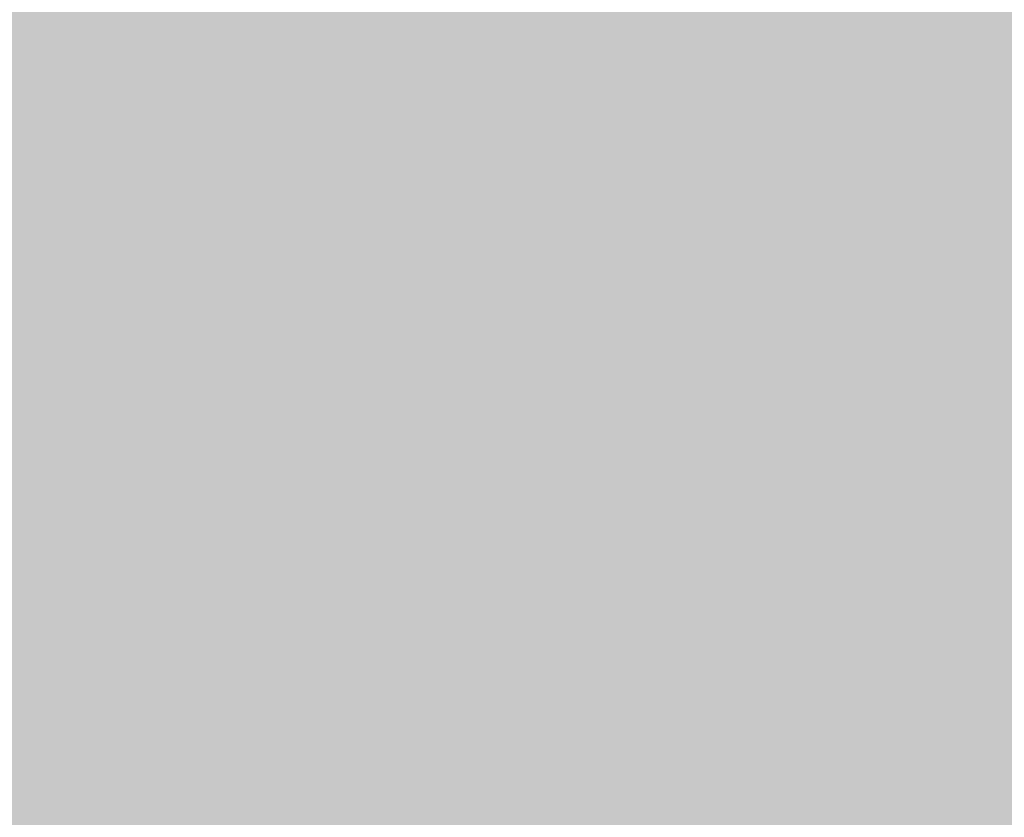
# Model space of a CAD drawing. Units: millimetres. Extents: x 0 to 2267, y 0 to 1823.
# Tile 131 of 256: x 1600.37 to 1611.04, y 1234.76 to 1243.41. Entities that reach past the tile are written whole.
import ezdxf

# ---------------------------------------------------------------- set-up
doc = ezdxf.new("R2010")
doc.units = ezdxf.units.MM
doc.header["$MEASUREMENT"] = 0
doc.layers.add('M-DIMS', color=2, linetype='Continuous', lineweight=25)
doc.layers.add('M-HATC', color=252, linetype='Continuous', lineweight=18)
doc.styles.get("Standard").update_dxf_attribs({"font": 'arial.ttf'})
doc.dimstyles.get("Standard").update_dxf_attribs({"dimtxt": 7, "dimasz": 4, "dimexe": 0.18, "dimexo": 0.0625, "dimgap": 0.09, "dimtad": 0, "dimdec": 0, "dimzin": 0, "dimdsep": 46, "dimtxsty": 'Standard', "dimcen": 0.09, "dimadec": 0, "dimazin": 0, "dimtfac": 1, "dimtdec": 0, "dimtofl": 0, "dimtmove": 0, "dimatfit": 3, "dimfxl": 1, "dimtolj": 1, "dimtzin": 0, "dimarcsym": 0})

# ---------------------------------------------------------------- blocks, each defined once
blk = doc.blocks.new('*D19')
at = {"layer": 'Defpoints', "color": 0, "transparency": 16777216}
for p in [(1605.34, 1483.304), (1445.529, 1333.885)]:
    blk.add_point(p, dxfattribs=at)
at = {"layer": 'M-DIMS', "color": 0, "lineweight": -2, "transparency": 16777216}
for p, q in [((1605.34, 1483.214), (1605.34, 1483.394)), ((1605.25, 1483.304), (1605.43, 1483.304)), ((1366.324, 1259.831), (1442.607, 1331.153))]:
    blk.add_line(p, q, dxfattribs=at)
at = {"layer": 'M-DIMS', "color": 0, "transparency": 16777216}
blk.add_solid([(1442.152, 1331.64), (1443.063, 1330.666), (1445.529, 1333.885)], dxfattribs=at)
at = {"layer": 'M-DIMS', "color": 0, "transparency": 16777216, "insert": (1349.643, 1244.233), "char_height": 7, "attachment_point": 5, "rotation": 43.0753}
blk.add_mtext('\\A1;2X R218.8', dxfattribs=at)

msp = doc.modelspace()

# ---------------------------------------------------------------- hatches: boundary and pattern name
at = {"layer": 'M-HATC'}
h = msp.add_hatch(color=256, dxfattribs=at)
h.dxf.hatch_style = 1
h.paths.add_polyline_path([(2065.771, 1618.062, 0.236068), (2055.771, 1638.062), (1381.087, 1638.062, 0.236068), (1371.087, 1618.062), (1371.087, 1603.062), (2055.771, 1603.062), (2065.771, 1603.062)])
h.paths.add_polyline_path([(2062.772, 1550.296), (2062.772, 1560.296), (1374.086, 1560.296), (1374.086, 1550.296), (1374.086, 1540.296), (1384.086, 1540.296), (1389.086, 1540.296), (2062.772, 1540.296)])
h.paths.add_polyline_path([(1930.929, 1282.766), (1505.929, 1282.766), (1587.628, 1235.597, 0.131652), (1600.128, 1232.247), (1836.73, 1232.247, 0.131652), (1849.23, 1235.597)])
h.paths.add_polyline_path([(1930.929, 1117.417), (1905.929, 1117.417), (1505.929, 1117.417), (1505.929, 1077.417), (1930.929, 1077.417)])
h = msp.add_hatch(color=256, dxfattribs=at)
h.dxf.hatch_style = 1
h.paths.add_polyline_path([(2055.771, 1603.062), (1381.087, 1603.062), (1381.087, 1598.062), (2055.771, 1598.062)])
h.paths.add_polyline_path([(2055.771, 1598.062), (1381.087, 1598.062), (1381.087, 1593.062), (2055.771, 1593.062)])
h.paths.add_polyline_path([(2051.307, 1536.761), (1385.55, 1536.761), (1385.55, 1526.761), (1387.55, 1526.761), (1388.537, 1525.053), (1385.332, 1521.233), (1385.332, 1521.223), (2050.254, 1522.749), (2048.321, 1525.053), (2049.307, 1526.761), (2051.307, 1526.761)])
edge = h.paths.add_edge_path()
edge.add_arc((1847.535, 1379.149), 135, 222.60306, 222.89085, ccw=False)
edge.add_line((1748.166, 1287.766), (1683.092, 1287.766))
edge.add_arc((1583.724, 1379.149), 135, 317.10915, 317.39694, ccw=False)
edge.add_arc((1678.969, 1290.671), 5, 222.8909, 317.1091, ccw=False)
edge.add_arc((1774.213, 1379.149), 135, 222.60306, 222.89085, ccw=False)
edge.add_line((1674.845, 1287.766), (1609.771, 1287.766))
edge.add_arc((1510.403, 1379.149), 135, 317.10915, 317.39694, ccw=False)
edge.add_arc((1605.647, 1290.671), 5, 222.8909, 317.1091, ccw=False)
edge.add_arc((1700.892, 1379.149), 135, 222.60306, 222.89085, ccw=False)
edge.add_line((1601.524, 1287.766), (1536.45, 1287.766))
edge.add_arc((1437.081, 1379.149), 135, 317.10915, 317.39694, ccw=False)
edge.add_arc((1532.326, 1290.671), 5, 222.8909, 317.1091, ccw=False)
edge.add_arc((1627.571, 1379.149), 135, 222.60306, 222.89085, ccw=False)
edge.add_line((1528.203, 1287.766), (1505.929, 1287.766))
edge.add_spline(control_points=[(1505.929, 1287.766), (1504.262, 1287.766), (1504.262, 1282.766), (1505.929, 1282.766)], knot_values=[0, 0, 0, 0, 5, 5, 5, 5], degree=3, periodic=0)
edge.add_line((1505.929, 1282.766), (1930.929, 1282.766))
edge.add_spline(control_points=[(1930.929, 1282.766), (1932.596, 1282.766), (1932.596, 1287.766), (1930.929, 1287.766)], knot_values=[0, 0, 0, 0, 5, 5, 5, 5], degree=3, periodic=0)
edge.add_line((1930.929, 1287.766), (1903.056, 1287.766))
edge.add_arc((1803.688, 1379.149), 135, 317.10915, 317.39694, ccw=False)
edge.add_arc((1898.932, 1290.671), 5, 222.8909, 317.1091, ccw=False)
edge.add_arc((1994.177, 1379.149), 135, 222.60306, 222.89085, ccw=False)
edge.add_line((1894.809, 1287.766), (1829.735, 1287.766))
edge.add_arc((1730.366, 1379.149), 135, 317.10915, 317.39694, ccw=False)
edge.add_arc((1825.611, 1290.671), 5, 222.8909, 317.1091, ccw=False)
edge.add_arc((1920.856, 1379.149), 135, 222.60306, 222.89085, ccw=False)
edge.add_line((1821.487, 1287.766), (1756.413, 1287.766))
edge.add_arc((1657.045, 1379.149), 135, 317.10915, 317.39694, ccw=False)
edge.add_arc((1752.29, 1290.671), 5, 222.8909, 317.1091, ccw=False)
edge = h.paths.add_edge_path()
edge.add_spline(control_points=[(1843.429, 1227.247), (1845.096, 1227.247), (1845.096, 1232.247), (1843.429, 1232.247)], knot_values=[0, 0, 0, 0, 5, 5, 5, 5], degree=3, periodic=0)
edge.add_line((1843.429, 1232.247), (1593.429, 1232.247))
edge.add_spline(control_points=[(1593.429, 1232.247), (1591.762, 1232.247), (1591.762, 1227.247), (1593.429, 1227.247)], knot_values=[0, 0, 0, 0, 5, 5, 5, 5], degree=3, periodic=0)
edge.add_line((1593.429, 1227.247), (1843.429, 1227.247))
h.paths.add_polyline_path([(1905.929, 1127.417), (1530.929, 1127.417, 0.414214), (1520.929, 1117.417), (1530.929, 1117.417), (1915.929, 1117.417, 0.414214)])
edge = h.paths.add_edge_path()
edge.add_arc((1397.086, 1498.408), 12.73, 90.7821, 190.8787, ccw=False)
edge.add_line((1396.912, 1511.136), (1428.01, 1511.349))
edge.add_line((1428.01, 1511.349), (1433.01, 1511.349))
edge.add_line((1433.01, 1511.349), (1434.439, 1511.349))
edge.add_arc((1419.474, 1498.08), 20, 41.561, 74.0821)
edge.add_line((1424.959, 1517.314), (1399.935, 1517.256))
edge.add_spline(control_points=[(1399.931, 1517.256), (1399.884, 1517.213), (1399.833, 1517.169), (1399.777, 1517.124)], knot_values=[11.567499, 11.567499, 11.567499, 11.567499, 11.814249, 11.814249, 11.814249, 11.814249], degree=3, periodic=0)
edge.add_spline(control_points=[(1399.633, 1517.01), (1399.583, 1516.972), (1399.531, 1516.934), (1399.476, 1516.895)], knot_values=[11.167718, 11.167718, 11.167718, 11.167718, 11.365188, 11.365188, 11.365188, 11.365188], degree=3, periodic=0)
edge.add_spline(control_points=[(1399.34, 1516.8), (1399.151, 1516.672), (1398.938, 1516.538), (1398.704, 1516.399)], knot_values=[10.376405, 10.376405, 10.376405, 10.376405, 11.00994, 11.00994, 11.00994, 11.00994], degree=3, periodic=0)
edge.add_spline(control_points=[(1398.657, 1516.372), (1398.579, 1516.326), (1398.498, 1516.28), (1398.415, 1516.233)], knot_values=[10.125175, 10.125175, 10.125175, 10.125175, 10.334406, 10.334406, 10.334406, 10.334406], degree=3, periodic=0)
edge.add_spline(control_points=[(1398.264, 1516.149), (1398.196, 1516.111), (1398.126, 1516.073), (1398.055, 1516.035)], knot_values=[9.832246, 9.832246, 9.832246, 9.832246, 9.999658, 9.999658, 9.999658, 9.999658], degree=3, periodic=0)
edge.add_spline(control_points=[(1397.999, 1516.005), (1397.731, 1515.862), (1397.446, 1515.717), (1397.147, 1515.571)], knot_values=[9.161808, 9.161808, 9.161808, 9.161808, 9.787769, 9.787769, 9.787769, 9.787769], degree=3, periodic=0)
edge.add_spline(control_points=[(1397.147, 1515.571), (1396.842, 1515.423), (1396.522, 1515.274), (1396.191, 1515.126)], knot_values=[8.524455, 8.524455, 8.524455, 8.524455, 9.161808, 9.161808, 9.161808, 9.161808], degree=3, periodic=0)
edge.add_spline(control_points=[(1396.078, 1515.076), (1395.985, 1515.035), (1395.892, 1514.994), (1395.798, 1514.953)], knot_values=[8.275193, 8.275193, 8.275193, 8.275193, 8.451726, 8.451726, 8.451726, 8.451726], degree=3, periodic=0)
edge.add_spline(control_points=[(1395.602, 1514.869), (1395.5, 1514.826), (1395.397, 1514.782), (1395.293, 1514.739)], knot_values=[7.962917, 7.962917, 7.962917, 7.962917, 8.152764, 8.152764, 8.152764, 8.152764], degree=3, periodic=0)
edge.add_spline(control_points=[(1395.212, 1514.706), (1394.828, 1514.547), (1394.435, 1514.393), (1394.036, 1514.244)], knot_values=[7.21254, 7.21254, 7.21254, 7.21254, 7.913148, 7.913148, 7.913148, 7.913148], degree=3, periodic=0)
edge.add_spline(control_points=[(1394.036, 1514.244), (1393.708, 1514.121), (1393.375, 1514.003), (1393.043, 1513.889)], knot_values=[6.633733, 6.633733, 6.633733, 6.633733, 7.21254, 7.21254, 7.21254, 7.21254], degree=3, periodic=0)
edge.add_spline(control_points=[(1392.821, 1513.815), (1392.72, 1513.781), (1392.618, 1513.748), (1392.517, 1513.715)], knot_values=[6.328796, 6.328796, 6.328796, 6.328796, 6.505493, 6.505493, 6.505493, 6.505493], degree=3, periodic=0)
edge.add_spline(control_points=[(1392.517, 1513.715), (1392.319, 1513.652), (1392.121, 1513.59), (1391.924, 1513.531)], knot_values=[5.984605, 5.984605, 5.984605, 5.984605, 6.328796, 6.328796, 6.328796, 6.328796], degree=3, periodic=0)
edge.add_spline(control_points=[(1391.792, 1513.491), (1391.312, 1513.35), (1390.838, 1513.224), (1390.378, 1513.117)], knot_values=[5.066697, 5.066697, 5.066697, 5.066697, 5.907055, 5.907055, 5.907055, 5.907055], degree=3, periodic=0)
edge.add_spline(control_points=[(1390.378, 1513.117), (1390.18, 1513.071), (1389.984, 1513.028), (1389.791, 1512.99)], knot_values=[4.70367, 4.70367, 4.70367, 4.70367, 5.066695, 5.066695, 5.066695, 5.066695], degree=3, periodic=0)
edge.add_spline(control_points=[(1389.422, 1512.92), (1389.246, 1512.889), (1389.073, 1512.862), (1388.904, 1512.838)], knot_values=[4.130571, 4.130571, 4.130571, 4.130571, 4.469816, 4.469816, 4.469816, 4.469816], degree=3, periodic=0)
edge.add_spline(control_points=[(1388.904, 1512.838), (1388.591, 1512.795), (1388.291, 1512.764), (1388.007, 1512.749)], knot_values=[3.504031, 3.504031, 3.504031, 3.504031, 4.130571, 4.130571, 4.130571, 4.130571], degree=3, periodic=0)
edge.add_spline(control_points=[(1387.936, 1512.746), (1387.854, 1512.742), (1387.773, 1512.74), (1387.694, 1512.739)], knot_values=[3.268866, 3.268866, 3.268866, 3.268866, 3.451164, 3.451164, 3.451164, 3.451164], degree=3, periodic=0)
edge.add_spline(control_points=[(1387.335, 1512.744), (1387.208, 1512.75), (1387.085, 1512.76), (1386.967, 1512.774)], knot_values=[2.670686, 2.670686, 2.670686, 2.670686, 2.984, 2.984, 2.984, 2.984], degree=3, periodic=0)
edge.add_spline(control_points=[(1386.833, 1512.792), (1386.821, 1512.794), (1386.809, 1512.796), (1386.797, 1512.798)], knot_values=[2.516981, 2.516981, 2.516981, 2.516981, 2.549528, 2.549528, 2.549528, 2.549528], degree=3, periodic=0)
edge.add_spline(control_points=[(1386.453, 1512.873), (1386.426, 1512.881), (1386.399, 1512.889), (1386.373, 1512.897)], knot_values=[2.095869, 2.095869, 2.095869, 2.095869, 2.17941, 2.17941, 2.17941, 2.17941], degree=3, periodic=0)
edge.add_spline(control_points=[(1386.069, 1513.019), (1386.063, 1513.022), (1386.058, 1513.025), (1386.052, 1513.028)], knot_values=[1.72453, 1.72453, 1.72453, 1.72453, 1.745933, 1.745933, 1.745933, 1.745933], degree=3, periodic=0)
edge.add_arc((1399.474, 1498.08), 20, 131.8243, 180)
edge.add_arc((1630.334, 1505.548), 250.971, 181.70518, 236.42798)
edge.add_arc((1605.34, 1483.304), 218.782, 238.66083, 243.34961)
edge.add_arc((1647.091, 1510.359), 262.899, 183.12984, 237.85344, ccw=False)
h.paths.add_polyline_path([(1406.537, 1391.964, 0.149382), (1491.551, 1296.442, -0.129517)], flags=17)
edge = h.paths.add_edge_path()
edge.add_arc((2037.384, 1498.08), 20, 0, 48.2659)
edge.add_spline(control_points=[(2050.697, 1513.005), (2050.651, 1512.985), (2050.603, 1512.966), (2050.554, 1512.948)], knot_values=[1.835652, 1.835652, 1.835652, 1.835652, 2.000781, 2.000781, 2.000781, 2.000781], degree=3, periodic=0)
edge.add_spline(control_points=[(2050.462, 1512.917), (2050.479, 1512.922), (2050.496, 1512.928), (2050.513, 1512.934)], knot_values=[2.045477, 2.045477, 2.045477, 2.045477, 2.101389, 2.101389, 2.101389, 2.101389], degree=3, periodic=0)
edge.add_spline(control_points=[(2050.129, 1512.834), (2050.198, 1512.847), (2050.266, 1512.862), (2050.331, 1512.879)], knot_values=[2.237629, 2.237629, 2.237629, 2.237629, 2.435841, 2.435841, 2.435841, 2.435841], degree=3, periodic=0)
edge.add_spline(control_points=[(2050.095, 1512.828), (2050.106, 1512.83), (2050.118, 1512.832), (2050.129, 1512.834)], knot_values=[2.435841, 2.435841, 2.435841, 2.435841, 2.468321, 2.468321, 2.468321, 2.468321], degree=3, periodic=0)
edge.add_spline(control_points=[(2049.784, 1512.785), (2049.855, 1512.792), (2049.924, 1512.801), (2049.992, 1512.811)], knot_values=[2.563852, 2.563852, 2.563852, 2.563852, 2.748541, 2.748541, 2.748541, 2.748541], degree=3, periodic=0)
edge.add_spline(control_points=[(2049.405, 1512.762), (2049.536, 1512.765), (2049.663, 1512.773), (2049.784, 1512.785)], knot_values=[2.748541, 2.748541, 2.748541, 2.748541, 3.064882, 3.064882, 3.064882, 3.064882], degree=3, periodic=0)
edge.add_spline(control_points=[(2049.17, 1512.76), (2049.234, 1512.759), (2049.297, 1512.759), (2049.358, 1512.761)], knot_values=[3.102309, 3.102309, 3.102309, 3.102309, 3.2503, 3.2503, 3.2503, 3.2503], degree=3, periodic=0)
edge.add_spline(control_points=[(2048.857, 1512.769), (2048.964, 1512.764), (2049.068, 1512.761), (2049.17, 1512.76)], knot_values=[3.2503, 3.2503, 3.2503, 3.2503, 3.486069, 3.486069, 3.486069, 3.486069], degree=3, periodic=0)
edge.add_spline(control_points=[(2048.692, 1512.779), (2048.373, 1512.801), (2048.035, 1512.841), (2047.682, 1512.897)], knot_values=[3.606429, 3.606429, 3.606429, 3.606429, 4.2989, 4.2989, 4.2989, 4.2989], degree=3, periodic=0)
edge.add_spline(control_points=[(2047.682, 1512.897), (2047.546, 1512.919), (2047.408, 1512.942), (2047.268, 1512.969)], knot_values=[4.2989, 4.2989, 4.2989, 4.2989, 4.565769, 4.565769, 4.565769, 4.565769], degree=3, periodic=0)
edge.add_spline(control_points=[(2047.268, 1512.969), (2047.145, 1512.991), (2047.021, 1513.016), (2046.895, 1513.042)], knot_values=[4.565769, 4.565769, 4.565769, 4.565769, 4.799971, 4.799971, 4.799971, 4.799971], degree=3, periodic=0)
edge.add_spline(control_points=[(2046.895, 1513.042), (2046.529, 1513.119), (2046.151, 1513.209), (2045.768, 1513.311)], knot_values=[4.799971, 4.799971, 4.799971, 4.799971, 5.483718, 5.483718, 5.483718, 5.483718], degree=3, periodic=0)
edge.add_spline(control_points=[(2045.768, 1513.311), (2045.372, 1513.415), (2044.97, 1513.532), (2044.566, 1513.659)], knot_values=[5.483718, 5.483718, 5.483718, 5.483718, 6.187866, 6.187866, 6.187866, 6.187866], degree=3, periodic=0)
edge.add_spline(control_points=[(2044.566, 1513.659), (2044.415, 1513.706), (2044.263, 1513.755), (2044.112, 1513.805)], knot_values=[6.187866, 6.187866, 6.187866, 6.187866, 6.451551, 6.451551, 6.451551, 6.451551], degree=3, periodic=0)
edge.add_spline(control_points=[(2044.112, 1513.805), (2043.997, 1513.843), (2043.882, 1513.881), (2043.767, 1513.92)], knot_values=[6.451551, 6.451551, 6.451551, 6.451551, 6.651434, 6.651434, 6.651434, 6.651434], degree=3, periodic=0)
edge.add_spline(control_points=[(2043.767, 1513.92), (2043.372, 1514.055), (2042.977, 1514.198), (2042.589, 1514.346)], knot_values=[6.651434, 6.651434, 6.651434, 6.651434, 7.338879, 7.338879, 7.338879, 7.338879], degree=3, periodic=0)
edge.add_spline(control_points=[(2042.589, 1514.346), (2042.164, 1514.507), (2041.746, 1514.675), (2041.341, 1514.846)], knot_values=[7.338879, 7.338879, 7.338879, 7.338879, 8.089209, 8.089209, 8.089209, 8.089209], degree=3, periodic=0)
edge.add_spline(control_points=[(2041.341, 1514.846), (2041.103, 1514.946), (2040.869, 1515.048), (2040.64, 1515.15)], knot_values=[8.089209, 8.089209, 8.089209, 8.089209, 8.529587, 8.529587, 8.529587, 8.529587], degree=3, periodic=0)
edge.add_spline(control_points=[(2040.51, 1515.209), (2040.082, 1515.402), (2039.675, 1515.597), (2039.295, 1515.789)], knot_values=[8.613818, 8.613818, 8.613818, 8.613818, 9.44571, 9.44571, 9.44571, 9.44571], degree=3, periodic=0)
edge.add_spline(control_points=[(2039.295, 1515.789), (2039.062, 1515.907), (2038.839, 1516.025), (2038.629, 1516.14)], knot_values=[9.44571, 9.44571, 9.44571, 9.44571, 9.956404, 9.956404, 9.956404, 9.956404], degree=3, periodic=0)
edge.add_spline(control_points=[(2038.629, 1516.14), (2038.519, 1516.2), (2038.412, 1516.26), (2038.309, 1516.319)], knot_values=[9.956404, 9.956404, 9.956404, 9.956404, 10.223542, 10.223542, 10.223542, 10.223542], degree=3, periodic=0)
edge.add_spline(control_points=[(2038.309, 1516.319), (2038.214, 1516.374), (2038.122, 1516.428), (2038.033, 1516.481)], knot_values=[10.223542, 10.223542, 10.223542, 10.223542, 10.47051, 10.47051, 10.47051, 10.47051], degree=3, periodic=0)
edge.add_spline(control_points=[(2038.033, 1516.481), (2037.786, 1516.63), (2037.564, 1516.773), (2037.372, 1516.909)], knot_values=[10.47051, 10.47051, 10.47051, 10.47051, 11.15767, 11.15767, 11.15767, 11.15767], degree=3, periodic=0)
edge.add_spline(control_points=[(2037.372, 1516.909), (2037.279, 1516.975), (2037.193, 1517.04), (2037.114, 1517.102)], knot_values=[11.15767, 11.15767, 11.15767, 11.15767, 11.49227, 11.49227, 11.49227, 11.49227], degree=3, periodic=0)
edge.add_spline(control_points=[(2036.856, 1517.326), (2036.915, 1517.269), (2036.981, 1517.21), (2037.056, 1517.149)], knot_values=[11.577341, 11.577341, 11.577341, 11.577341, 11.91035, 11.91035, 11.91035, 11.91035], degree=3, periodic=0)
edge.add_spline(control_points=[(2036.807, 1517.375), (2036.823, 1517.359), (2036.839, 1517.342), (2036.856, 1517.326)], knot_values=[11.91035, 11.91035, 11.91035, 11.91035, 12.007402, 12.007402, 12.007402, 12.007402], degree=3, periodic=0)
edge.add_spline(control_points=[(2036.702, 1517.494), (2036.71, 1517.483), (2036.72, 1517.472), (2036.729, 1517.461)], knot_values=[12.184155, 12.184155, 12.184155, 12.184155, 12.255409, 12.255409, 12.255409, 12.255409], degree=3, periodic=0)
edge.add_spline(control_points=[(2036.616, 1517.621), (2036.62, 1517.613), (2036.624, 1517.606), (2036.629, 1517.598)], knot_values=[12.487913, 12.487913, 12.487913, 12.487913, 12.541035, 12.541035, 12.541035, 12.541035], degree=3, periodic=0)
edge.add_spline(control_points=[(2036.563, 1517.786), (2036.564, 1517.779), (2036.564, 1517.773), (2036.565, 1517.766)], knot_values=[12.911761, 12.911761, 12.911761, 12.911761, 12.968286, 12.968286, 12.968286, 12.968286], degree=3, periodic=0)
edge.add_spline(control_points=[(2036.617, 1517.93), (2036.612, 1517.926), (2036.609, 1517.921), (2036.605, 1517.916)], knot_values=[13.382527, 13.382527, 13.382527, 13.382527, 13.433791, 13.433791, 13.433791, 13.433791], degree=3, periodic=0)
edge.add_spline(control_points=[(2036.749, 1518.017), (2036.736, 1518.012), (2036.724, 1518.006), (2036.712, 1518)], knot_values=[13.726299, 13.726299, 13.726299, 13.726299, 13.809928, 13.809928, 13.809928, 13.809928], degree=3, periodic=0)
edge.add_spline(control_points=[(2036.86, 1518.053), (2036.839, 1518.047), (2036.818, 1518.042), (2036.799, 1518.035)], knot_values=[13.910887, 13.910887, 13.910887, 13.910887, 14.02153, 14.02153, 14.02153, 14.02153], degree=3, periodic=0)
edge.add_line((2036.964, 1518.08), (2032.384, 1518.08))
edge.add_line((2032.384, 1518.08), (2027.384, 1518.08))
edge.add_line((2027.384, 1518.08), (2022.384, 1518.08))
edge.add_line((2022.384, 1518.08), (2017.384, 1518.08))
edge.add_arc((2017.384, 1498.08), 20, 90, 138.439)
edge.add_line((2002.419, 1511.349), (2003.848, 1511.349))
edge.add_line((2003.848, 1511.349), (2008.848, 1511.349))
edge.add_line((2008.848, 1511.349), (2039.772, 1511.138))
edge.add_arc((2039.772, 1498.408), 12.73, -10.8787, 90, ccw=False)
edge.add_arc((1789.767, 1510.359), 262.899, 302.14656, 356.87016, ccw=False)
edge.add_arc((1831.518, 1483.304), 218.782, 296.65039, 301.33917)
edge.add_arc((1806.524, 1505.548), 250.971, 303.57202, 358.29482)
h.paths.add_polyline_path([(2030.321, 1391.964, -0.129517), (1945.307, 1296.442, 0.149382)], flags=17)
edge = h.paths.add_edge_path()
edge.add_spline(control_points=[(2037.246, 1518.082), (2037.29, 1518.081), (2037.336, 1518.08), (2037.384, 1518.08)], knot_values=[0.000012, 0.000012, 0.000012, 0.000012, 0.144754, 0.144754, 0.144754, 0.144754], degree=3, periodic=0)
edge.add_line((2037.336, 1518.08), (2037.01, 1518.08))
edge.add_spline(control_points=[(2037.01, 1518.08), (2036.982, 1518.077), (2036.956, 1518.073), (2036.931, 1518.068)], knot_values=[14.13465, 14.13465, 14.13465, 14.13465, 14.247197, 14.247197, 14.247197, 14.247197], degree=3, periodic=0)
edge.add_spline(control_points=[(2036.931, 1518.068), (2036.928, 1518.067), (2036.924, 1518.067), (2036.921, 1518.066)], knot_values=[14.118315, 14.118315, 14.118315, 14.118315, 14.13465, 14.13465, 14.13465, 14.13465], degree=3, periodic=0)
edge.add_spline(control_points=[(2036.921, 1518.066), (2036.912, 1518.064), (2036.903, 1518.063), (2036.895, 1518.061)], knot_values=[14.078086, 14.078086, 14.078086, 14.078086, 14.118315, 14.118315, 14.118315, 14.118315], degree=3, periodic=0)
edge.add_spline(control_points=[(2036.895, 1518.061), (2036.883, 1518.058), (2036.872, 1518.056), (2036.86, 1518.053)], knot_values=[14.02153, 14.02153, 14.02153, 14.02153, 14.078086, 14.078086, 14.078086, 14.078086], degree=3, periodic=0)
edge.add_spline(control_points=[(2036.86, 1518.053), (2036.839, 1518.047), (2036.818, 1518.042), (2036.799, 1518.035)], knot_values=[13.910887, 13.910887, 13.910887, 13.910887, 14.02153, 14.02153, 14.02153, 14.02153], degree=3, periodic=0)
edge.add_spline(control_points=[(2036.799, 1518.035), (2036.798, 1518.035), (2036.797, 1518.035), (2036.797, 1518.035)], knot_values=[13.906906, 13.906906, 13.906906, 13.906906, 13.910887, 13.910887, 13.910887, 13.910887], degree=3, periodic=0)
edge.add_spline(control_points=[(2036.797, 1518.035), (2036.788, 1518.032), (2036.78, 1518.029), (2036.772, 1518.026)], knot_values=[13.857826, 13.857826, 13.857826, 13.857826, 13.906906, 13.906906, 13.906906, 13.906906], degree=3, periodic=0)
edge.add_spline(control_points=[(2036.772, 1518.026), (2036.764, 1518.023), (2036.756, 1518.02), (2036.749, 1518.017)], knot_values=[13.809928, 13.809928, 13.809928, 13.809928, 13.857826, 13.857826, 13.857826, 13.857826], degree=3, periodic=0)
edge.add_spline(control_points=[(2036.749, 1518.017), (2036.736, 1518.012), (2036.724, 1518.006), (2036.712, 1518)], knot_values=[13.726299, 13.726299, 13.726299, 13.726299, 13.809928, 13.809928, 13.809928, 13.809928], degree=3, periodic=0)
edge.add_spline(control_points=[(2036.712, 1518), (2036.712, 1518), (2036.712, 1518), (2036.711, 1518)], knot_values=[13.723993, 13.723993, 13.723993, 13.723993, 13.726299, 13.726299, 13.726299, 13.726299], degree=3, periodic=0)
edge.add_spline(control_points=[(2036.711, 1518), (2036.706, 1517.997), (2036.701, 1517.994), (2036.696, 1517.992)], knot_values=[13.686536, 13.686536, 13.686536, 13.686536, 13.723993, 13.723993, 13.723993, 13.723993], degree=3, periodic=0)
edge.add_spline(control_points=[(2036.696, 1517.992), (2036.692, 1517.989), (2036.687, 1517.987), (2036.683, 1517.984)], knot_values=[13.651251, 13.651251, 13.651251, 13.651251, 13.686536, 13.686536, 13.686536, 13.686536], degree=3, periodic=0)
edge.add_spline(control_points=[(2036.683, 1517.984), (2036.676, 1517.98), (2036.67, 1517.976), (2036.664, 1517.971)], knot_values=[13.596804, 13.596804, 13.596804, 13.596804, 13.651251, 13.651251, 13.651251, 13.651251], degree=3, periodic=0)
edge.add_spline(control_points=[(2036.664, 1517.971), (2036.664, 1517.971), (2036.663, 1517.971), (2036.663, 1517.971)], knot_values=[13.593956, 13.593956, 13.593956, 13.593956, 13.596804, 13.596804, 13.596804, 13.596804], degree=3, periodic=0)
edge.add_spline(control_points=[(2036.663, 1517.971), (2036.66, 1517.969), (2036.658, 1517.967), (2036.655, 1517.965)], knot_values=[13.570322, 13.570322, 13.570322, 13.570322, 13.593956, 13.593956, 13.593956, 13.593956], degree=3, periodic=0)
edge.add_spline(control_points=[(2036.655, 1517.965), (2036.653, 1517.963), (2036.65, 1517.961), (2036.647, 1517.959)], knot_values=[13.545477, 13.545477, 13.545477, 13.545477, 13.570322, 13.570322, 13.570322, 13.570322], degree=3, periodic=0)
edge.add_spline(control_points=[(2036.647, 1517.959), (2036.647, 1517.959), (2036.647, 1517.959), (2036.647, 1517.959)], knot_values=[13.543931, 13.543931, 13.543931, 13.543931, 13.545477, 13.545477, 13.545477, 13.545477], degree=3, periodic=0)
edge.add_spline(control_points=[(2036.647, 1517.959), (2036.641, 1517.954), (2036.636, 1517.949), (2036.631, 1517.945)], knot_values=[13.488237, 13.488237, 13.488237, 13.488237, 13.543931, 13.543931, 13.543931, 13.543931], degree=3, periodic=0)
edge.add_spline(control_points=[(2036.631, 1517.945), (2036.628, 1517.942), (2036.626, 1517.94), (2036.623, 1517.937)], knot_values=[13.460307, 13.460307, 13.460307, 13.460307, 13.488237, 13.488237, 13.488237, 13.488237], degree=3, periodic=0)
edge.add_spline(control_points=[(2036.623, 1517.937), (2036.622, 1517.936), (2036.62, 1517.934), (2036.618, 1517.932)], knot_values=[13.439712, 13.439712, 13.439712, 13.439712, 13.460307, 13.460307, 13.460307, 13.460307], degree=3, periodic=0)
edge.add_spline(control_points=[(2036.618, 1517.932), (2036.618, 1517.931), (2036.617, 1517.931), (2036.617, 1517.93)], knot_values=[13.433791, 13.433791, 13.433791, 13.433791, 13.439712, 13.439712, 13.439712, 13.439712], degree=3, periodic=0)
edge.add_spline(control_points=[(2036.617, 1517.93), (2036.612, 1517.926), (2036.609, 1517.921), (2036.605, 1517.916)], knot_values=[13.382527, 13.382527, 13.382527, 13.382527, 13.433791, 13.433791, 13.433791, 13.433791], degree=3, periodic=0)
edge.add_spline(control_points=[(2036.605, 1517.916), (2036.603, 1517.913), (2036.6, 1517.91), (2036.598, 1517.907)], knot_values=[13.350017, 13.350017, 13.350017, 13.350017, 13.382527, 13.382527, 13.382527, 13.382527], degree=3, periodic=0)
edge.add_spline(control_points=[(2036.598, 1517.907), (2036.597, 1517.906), (2036.596, 1517.904), (2036.595, 1517.903)], knot_values=[13.333922, 13.333922, 13.333922, 13.333922, 13.350017, 13.350017, 13.350017, 13.350017], degree=3, periodic=0)
edge.add_spline(control_points=[(2036.595, 1517.903), (2036.595, 1517.902), (2036.594, 1517.901), (2036.593, 1517.9)], knot_values=[13.323828, 13.323828, 13.323828, 13.323828, 13.333922, 13.333922, 13.333922, 13.333922], degree=3, periodic=0)
edge.add_spline(control_points=[(2036.593, 1517.9), (2036.59, 1517.895), (2036.588, 1517.891), (2036.585, 1517.886)], knot_values=[13.277545, 13.277545, 13.277545, 13.277545, 13.323828, 13.323828, 13.323828, 13.323828], degree=3, periodic=0)
edge.add_spline(control_points=[(2036.585, 1517.886), (2036.584, 1517.883), (2036.582, 1517.879), (2036.58, 1517.875)], knot_values=[13.240119, 13.240119, 13.240119, 13.240119, 13.277545, 13.277545, 13.277545, 13.277545], degree=3, periodic=0)
edge.add_spline(control_points=[(2036.58, 1517.875), (2036.58, 1517.874), (2036.579, 1517.873), (2036.578, 1517.872)], knot_values=[13.228211, 13.228211, 13.228211, 13.228211, 13.240119, 13.240119, 13.240119, 13.240119], degree=3, periodic=0)
edge.add_spline(control_points=[(2036.578, 1517.872), (2036.578, 1517.87), (2036.577, 1517.869), (2036.577, 1517.868)], knot_values=[13.215717, 13.215717, 13.215717, 13.215717, 13.228211, 13.228211, 13.228211, 13.228211], degree=3, periodic=0)
edge.add_spline(control_points=[(2036.577, 1517.868), (2036.575, 1517.864), (2036.574, 1517.86), (2036.573, 1517.857)], knot_values=[13.179847, 13.179847, 13.179847, 13.179847, 13.215717, 13.215717, 13.215717, 13.215717], degree=3, periodic=0)
edge.add_spline(control_points=[(2036.573, 1517.857), (2036.571, 1517.851), (2036.57, 1517.846), (2036.569, 1517.841)], knot_values=[13.132017, 13.132017, 13.132017, 13.132017, 13.179847, 13.179847, 13.179847, 13.179847], degree=3, periodic=0)
edge.add_spline(control_points=[(2036.569, 1517.841), (2036.568, 1517.84), (2036.568, 1517.839), (2036.568, 1517.838)], knot_values=[13.122482, 13.122482, 13.122482, 13.122482, 13.132017, 13.132017, 13.132017, 13.132017], degree=3, periodic=0)
edge.add_spline(control_points=[(2036.568, 1517.838), (2036.568, 1517.836), (2036.567, 1517.835), (2036.567, 1517.833)], knot_values=[13.105592, 13.105592, 13.105592, 13.105592, 13.122482, 13.122482, 13.122482, 13.122482], degree=3, periodic=0)
edge.add_spline(control_points=[(2036.567, 1517.833), (2036.566, 1517.829), (2036.566, 1517.826), (2036.565, 1517.822)], knot_values=[13.074063, 13.074063, 13.074063, 13.074063, 13.105592, 13.105592, 13.105592, 13.105592], degree=3, periodic=0)
edge.add_spline(control_points=[(2036.565, 1517.822), (2036.565, 1517.822), (2036.565, 1517.822), (2036.565, 1517.822)], knot_values=[13.074043, 13.074043, 13.074043, 13.074043, 13.074063, 13.074063, 13.074063, 13.074063], degree=3, periodic=0)
edge.add_spline(control_points=[(2036.565, 1517.822), (2036.564, 1517.816), (2036.564, 1517.811), (2036.564, 1517.805)], knot_values=[13.021884, 13.021884, 13.021884, 13.021884, 13.074043, 13.074043, 13.074043, 13.074043], degree=3, periodic=0)
edge.add_spline(control_points=[(2036.564, 1517.805), (2036.564, 1517.804), (2036.564, 1517.803), (2036.564, 1517.803)], knot_values=[13.01674, 13.01674, 13.01674, 13.01674, 13.021884, 13.021884, 13.021884, 13.021884], degree=3, periodic=0)
edge.add_spline(control_points=[(2036.564, 1517.803), (2036.563, 1517.801), (2036.563, 1517.798), (2036.563, 1517.796)], knot_values=[12.996438, 12.996438, 12.996438, 12.996438, 13.01674, 13.01674, 13.01674, 13.01674], degree=3, periodic=0)
edge.add_spline(control_points=[(2036.563, 1517.796), (2036.563, 1517.793), (2036.563, 1517.789), (2036.563, 1517.786)], knot_values=[12.968286, 12.968286, 12.968286, 12.968286, 12.996438, 12.996438, 12.996438, 12.996438], degree=3, periodic=0)
edge.add_spline(control_points=[(2036.563, 1517.786), (2036.564, 1517.779), (2036.564, 1517.773), (2036.565, 1517.766)], knot_values=[12.911761, 12.911761, 12.911761, 12.911761, 12.968286, 12.968286, 12.968286, 12.968286], degree=3, periodic=0)
edge.add_spline(control_points=[(2036.565, 1517.766), (2036.565, 1517.766), (2036.565, 1517.766), (2036.565, 1517.766)], knot_values=[12.911017, 12.911017, 12.911017, 12.911017, 12.911761, 12.911761, 12.911761, 12.911761], degree=3, periodic=0)
edge.add_spline(control_points=[(2036.565, 1517.766), (2036.565, 1517.762), (2036.566, 1517.759), (2036.566, 1517.756)], knot_values=[12.88528, 12.88528, 12.88528, 12.88528, 12.911017, 12.911017, 12.911017, 12.911017], degree=3, periodic=0)
edge.add_spline(control_points=[(2036.566, 1517.756), (2036.567, 1517.753), (2036.567, 1517.751), (2036.568, 1517.748)], knot_values=[12.862519, 12.862519, 12.862519, 12.862519, 12.88528, 12.88528, 12.88528, 12.88528], degree=3, periodic=0)
edge.add_spline(control_points=[(2036.568, 1517.748), (2036.568, 1517.747), (2036.568, 1517.747), (2036.568, 1517.746)], knot_values=[12.858885, 12.858885, 12.858885, 12.858885, 12.862519, 12.862519, 12.862519, 12.862519], degree=3, periodic=0)
edge.add_spline(control_points=[(2036.568, 1517.746), (2036.569, 1517.74), (2036.571, 1517.733), (2036.572, 1517.726)], knot_values=[12.8053, 12.8053, 12.8053, 12.8053, 12.858885, 12.858885, 12.858885, 12.858885], degree=3, periodic=0)
edge.add_spline(control_points=[(2036.572, 1517.726), (2036.573, 1517.723), (2036.574, 1517.719), (2036.576, 1517.715)], knot_values=[12.775176, 12.775176, 12.775176, 12.775176, 12.8053, 12.8053, 12.8053, 12.8053], degree=3, periodic=0)
edge.add_spline(control_points=[(2036.576, 1517.715), (2036.576, 1517.713), (2036.577, 1517.71), (2036.578, 1517.708)], knot_values=[12.756759, 12.756759, 12.756759, 12.756759, 12.775176, 12.775176, 12.775176, 12.775176], degree=3, periodic=0)
edge.add_spline(control_points=[(2036.578, 1517.708), (2036.578, 1517.707), (2036.578, 1517.706), (2036.579, 1517.705)], knot_values=[12.748742, 12.748742, 12.748742, 12.748742, 12.756759, 12.756759, 12.756759, 12.756759], degree=3, periodic=0)
edge.add_spline(control_points=[(2036.579, 1517.705), (2036.581, 1517.698), (2036.583, 1517.692), (2036.586, 1517.685)], knot_values=[12.69959, 12.69959, 12.69959, 12.69959, 12.748742, 12.748742, 12.748742, 12.748742], degree=3, periodic=0)
edge.add_spline(control_points=[(2036.586, 1517.685), (2036.588, 1517.68), (2036.59, 1517.675), (2036.592, 1517.669)], knot_values=[12.659038, 12.659038, 12.659038, 12.659038, 12.69959, 12.69959, 12.69959, 12.69959], degree=3, periodic=0)
edge.add_spline(control_points=[(2036.592, 1517.669), (2036.594, 1517.665), (2036.596, 1517.66), (2036.598, 1517.656)], knot_values=[12.626806, 12.626806, 12.626806, 12.626806, 12.659038, 12.659038, 12.659038, 12.659038], degree=3, periodic=0)
edge.add_spline(control_points=[(2036.598, 1517.656), (2036.598, 1517.655), (2036.599, 1517.654), (2036.599, 1517.653)], knot_values=[12.619394, 12.619394, 12.619394, 12.619394, 12.626806, 12.626806, 12.626806, 12.626806], degree=3, periodic=0)
edge.add_spline(control_points=[(2036.599, 1517.653), (2036.604, 1517.642), (2036.61, 1517.632), (2036.616, 1517.621)], knot_values=[12.541039, 12.541039, 12.541039, 12.541039, 12.619394, 12.619394, 12.619394, 12.619394], degree=3, periodic=0)
edge.add_spline(control_points=[(2036.616, 1517.621), (2036.616, 1517.621), (2036.616, 1517.621), (2036.616, 1517.621)], knot_values=[12.541035, 12.541035, 12.541035, 12.541035, 12.541039, 12.541039, 12.541039, 12.541039], degree=3, periodic=0)
edge.add_spline(control_points=[(2036.616, 1517.621), (2036.62, 1517.613), (2036.624, 1517.606), (2036.629, 1517.598)], knot_values=[12.487913, 12.487913, 12.487913, 12.487913, 12.541035, 12.541035, 12.541035, 12.541035], degree=3, periodic=0)
edge.add_spline(control_points=[(2036.629, 1517.598), (2036.633, 1517.592), (2036.637, 1517.585), (2036.641, 1517.579)], knot_values=[12.443982, 12.443982, 12.443982, 12.443982, 12.487913, 12.487913, 12.487913, 12.487913], degree=3, periodic=0)
edge.add_spline(control_points=[(2036.641, 1517.579), (2036.641, 1517.578), (2036.642, 1517.576), (2036.643, 1517.575)], knot_values=[12.434996, 12.434996, 12.434996, 12.434996, 12.443982, 12.443982, 12.443982, 12.443982], degree=3, periodic=0)
edge.add_spline(control_points=[(2036.643, 1517.575), (2036.653, 1517.56), (2036.664, 1517.544), (2036.676, 1517.528)], knot_values=[12.329647, 12.329647, 12.329647, 12.329647, 12.434996, 12.434996, 12.434996, 12.434996], degree=3, periodic=0)
edge.add_spline(control_points=[(2036.676, 1517.528), (2036.684, 1517.517), (2036.693, 1517.505), (2036.702, 1517.494)], knot_values=[12.255409, 12.255409, 12.255409, 12.255409, 12.329647, 12.329647, 12.329647, 12.329647], degree=3, periodic=0)
edge.add_spline(control_points=[(2036.702, 1517.494), (2036.71, 1517.483), (2036.72, 1517.472), (2036.729, 1517.461)], knot_values=[12.184155, 12.184155, 12.184155, 12.184155, 12.255409, 12.255409, 12.255409, 12.255409], degree=3, periodic=0)
edge.add_spline(control_points=[(2036.729, 1517.461), (2036.744, 1517.444), (2036.759, 1517.426), (2036.775, 1517.409)], knot_values=[12.075961, 12.075961, 12.075961, 12.075961, 12.184155, 12.184155, 12.184155, 12.184155], degree=3, periodic=0)
edge.add_spline(control_points=[(2036.775, 1517.409), (2036.776, 1517.407), (2036.777, 1517.406), (2036.778, 1517.405)], knot_values=[12.069502, 12.069502, 12.069502, 12.069502, 12.075961, 12.075961, 12.075961, 12.075961], degree=3, periodic=0)
edge.add_spline(control_points=[(2036.778, 1517.405), (2036.788, 1517.395), (2036.797, 1517.385), (2036.807, 1517.375)], knot_values=[12.007402, 12.007402, 12.007402, 12.007402, 12.069502, 12.069502, 12.069502, 12.069502], degree=3, periodic=0)
edge.add_spline(control_points=[(2036.807, 1517.375), (2036.823, 1517.359), (2036.839, 1517.342), (2036.856, 1517.326)], knot_values=[11.91035, 11.91035, 11.91035, 11.91035, 12.007402, 12.007402, 12.007402, 12.007402], degree=3, periodic=0)
edge.add_spline(control_points=[(2036.856, 1517.326), (2036.915, 1517.269), (2036.981, 1517.21), (2037.056, 1517.149)], knot_values=[11.577341, 11.577341, 11.577341, 11.577341, 11.91035, 11.91035, 11.91035, 11.91035], degree=3, periodic=0)
edge.add_spline(control_points=[(2037.056, 1517.149), (2037.075, 1517.134), (2037.094, 1517.118), (2037.114, 1517.102)], knot_values=[11.49227, 11.49227, 11.49227, 11.49227, 11.577341, 11.577341, 11.577341, 11.577341], degree=3, periodic=0)
edge.add_spline(control_points=[(2037.114, 1517.102), (2037.193, 1517.04), (2037.279, 1516.975), (2037.372, 1516.909)], knot_values=[11.15767, 11.15767, 11.15767, 11.15767, 11.49227, 11.49227, 11.49227, 11.49227], degree=3, periodic=0)
edge.add_spline(control_points=[(2037.372, 1516.909), (2037.564, 1516.773), (2037.786, 1516.63), (2038.033, 1516.481)], knot_values=[10.47051, 10.47051, 10.47051, 10.47051, 11.15767, 11.15767, 11.15767, 11.15767], degree=3, periodic=0)
edge.add_spline(control_points=[(2038.033, 1516.481), (2038.122, 1516.428), (2038.214, 1516.374), (2038.309, 1516.319)], knot_values=[10.223542, 10.223542, 10.223542, 10.223542, 10.47051, 10.47051, 10.47051, 10.47051], degree=3, periodic=0)
edge.add_spline(control_points=[(2038.309, 1516.319), (2038.412, 1516.26), (2038.519, 1516.2), (2038.629, 1516.14)], knot_values=[9.956404, 9.956404, 9.956404, 9.956404, 10.223542, 10.223542, 10.223542, 10.223542], degree=3, periodic=0)
edge.add_spline(control_points=[(2038.629, 1516.14), (2038.839, 1516.025), (2039.062, 1515.907), (2039.295, 1515.789)], knot_values=[9.44571, 9.44571, 9.44571, 9.44571, 9.956404, 9.956404, 9.956404, 9.956404], degree=3, periodic=0)
edge.add_spline(control_points=[(2039.295, 1515.789), (2039.675, 1515.597), (2040.082, 1515.402), (2040.51, 1515.209)], knot_values=[8.613818, 8.613818, 8.613818, 8.613818, 9.44571, 9.44571, 9.44571, 9.44571], degree=3, periodic=0)
edge.add_spline(control_points=[(2040.51, 1515.209), (2040.553, 1515.189), (2040.597, 1515.17), (2040.64, 1515.15)], knot_values=[8.529587, 8.529587, 8.529587, 8.529587, 8.613818, 8.613818, 8.613818, 8.613818], degree=3, periodic=0)
edge.add_spline(control_points=[(2040.64, 1515.15), (2040.869, 1515.048), (2041.103, 1514.946), (2041.341, 1514.846)], knot_values=[8.089209, 8.089209, 8.089209, 8.089209, 8.529587, 8.529587, 8.529587, 8.529587], degree=3, periodic=0)
edge.add_spline(control_points=[(2041.341, 1514.846), (2041.746, 1514.675), (2042.164, 1514.507), (2042.589, 1514.346)], knot_values=[7.338879, 7.338879, 7.338879, 7.338879, 8.089209, 8.089209, 8.089209, 8.089209], degree=3, periodic=0)
edge.add_spline(control_points=[(2042.589, 1514.346), (2042.977, 1514.198), (2043.372, 1514.055), (2043.767, 1513.92)], knot_values=[6.651434, 6.651434, 6.651434, 6.651434, 7.338879, 7.338879, 7.338879, 7.338879], degree=3, periodic=0)
edge.add_spline(control_points=[(2043.767, 1513.92), (2043.882, 1513.881), (2043.997, 1513.843), (2044.112, 1513.805)], knot_values=[6.451551, 6.451551, 6.451551, 6.451551, 6.651434, 6.651434, 6.651434, 6.651434], degree=3, periodic=0)
edge.add_spline(control_points=[(2044.112, 1513.805), (2044.263, 1513.755), (2044.415, 1513.706), (2044.566, 1513.659)], knot_values=[6.187866, 6.187866, 6.187866, 6.187866, 6.451551, 6.451551, 6.451551, 6.451551], degree=3, periodic=0)
edge.add_spline(control_points=[(2044.566, 1513.659), (2044.97, 1513.532), (2045.372, 1513.415), (2045.768, 1513.311)], knot_values=[5.483718, 5.483718, 5.483718, 5.483718, 6.187866, 6.187866, 6.187866, 6.187866], degree=3, periodic=0)
edge.add_spline(control_points=[(2045.768, 1513.311), (2046.151, 1513.209), (2046.529, 1513.119), (2046.895, 1513.042)], knot_values=[4.799971, 4.799971, 4.799971, 4.799971, 5.483718, 5.483718, 5.483718, 5.483718], degree=3, periodic=0)
edge.add_spline(control_points=[(2046.895, 1513.042), (2047.021, 1513.016), (2047.145, 1512.991), (2047.268, 1512.969)], knot_values=[4.565769, 4.565769, 4.565769, 4.565769, 4.799971, 4.799971, 4.799971, 4.799971], degree=3, periodic=0)
edge.add_spline(control_points=[(2047.268, 1512.969), (2047.408, 1512.942), (2047.546, 1512.919), (2047.682, 1512.897)], knot_values=[4.2989, 4.2989, 4.2989, 4.2989, 4.565769, 4.565769, 4.565769, 4.565769], degree=3, periodic=0)
edge.add_spline(control_points=[(2047.682, 1512.897), (2048.035, 1512.841), (2048.373, 1512.801), (2048.692, 1512.779)], knot_values=[3.606429, 3.606429, 3.606429, 3.606429, 4.2989, 4.2989, 4.2989, 4.2989], degree=3, periodic=0)
edge.add_spline(control_points=[(2048.692, 1512.779), (2048.748, 1512.775), (2048.803, 1512.772), (2048.857, 1512.769)], knot_values=[3.486069, 3.486069, 3.486069, 3.486069, 3.606429, 3.606429, 3.606429, 3.606429], degree=3, periodic=0)
edge.add_spline(control_points=[(2048.857, 1512.769), (2048.964, 1512.764), (2049.068, 1512.761), (2049.17, 1512.76)], knot_values=[3.2503, 3.2503, 3.2503, 3.2503, 3.486069, 3.486069, 3.486069, 3.486069], degree=3, periodic=0)
edge.add_spline(control_points=[(2049.17, 1512.76), (2049.234, 1512.759), (2049.297, 1512.759), (2049.358, 1512.761)], knot_values=[3.102309, 3.102309, 3.102309, 3.102309, 3.2503, 3.2503, 3.2503, 3.2503], degree=3, periodic=0)
edge.add_spline(control_points=[(2049.358, 1512.761), (2049.374, 1512.761), (2049.39, 1512.761), (2049.405, 1512.762)], knot_values=[3.064882, 3.064882, 3.064882, 3.064882, 3.102309, 3.102309, 3.102309, 3.102309], degree=3, periodic=0)
edge.add_spline(control_points=[(2049.405, 1512.762), (2049.536, 1512.765), (2049.663, 1512.773), (2049.784, 1512.785)], knot_values=[2.748541, 2.748541, 2.748541, 2.748541, 3.064882, 3.064882, 3.064882, 3.064882], degree=3, periodic=0)
edge.add_spline(control_points=[(2049.784, 1512.785), (2049.855, 1512.792), (2049.924, 1512.801), (2049.992, 1512.811)], knot_values=[2.563852, 2.563852, 2.563852, 2.563852, 2.748541, 2.748541, 2.748541, 2.748541], degree=3, periodic=0)
edge.add_spline(control_points=[(2049.992, 1512.811), (2050.026, 1512.816), (2050.061, 1512.822), (2050.095, 1512.828)], knot_values=[2.468321, 2.468321, 2.468321, 2.468321, 2.563852, 2.563852, 2.563852, 2.563852], degree=3, periodic=0)
edge.add_spline(control_points=[(2050.095, 1512.828), (2050.106, 1512.83), (2050.118, 1512.832), (2050.129, 1512.834)], knot_values=[2.435841, 2.435841, 2.435841, 2.435841, 2.468321, 2.468321, 2.468321, 2.468321], degree=3, periodic=0)
edge.add_spline(control_points=[(2050.129, 1512.834), (2050.198, 1512.847), (2050.266, 1512.862), (2050.331, 1512.879)], knot_values=[2.237629, 2.237629, 2.237629, 2.237629, 2.435841, 2.435841, 2.435841, 2.435841], degree=3, periodic=0)
edge.add_spline(control_points=[(2050.331, 1512.879), (2050.375, 1512.891), (2050.419, 1512.903), (2050.462, 1512.917)], knot_values=[2.101389, 2.101389, 2.101389, 2.101389, 2.237629, 2.237629, 2.237629, 2.237629], degree=3, periodic=0)
edge.add_spline(control_points=[(2050.462, 1512.917), (2050.479, 1512.922), (2050.496, 1512.928), (2050.513, 1512.934)], knot_values=[2.045477, 2.045477, 2.045477, 2.045477, 2.101389, 2.101389, 2.101389, 2.101389], degree=3, periodic=0)
edge.add_spline(control_points=[(2050.513, 1512.934), (2050.527, 1512.938), (2050.54, 1512.943), (2050.554, 1512.948)], knot_values=[2.000781, 2.000781, 2.000781, 2.000781, 2.045477, 2.045477, 2.045477, 2.045477], degree=3, periodic=0)
edge.add_spline(control_points=[(2050.554, 1512.948), (2050.603, 1512.966), (2050.651, 1512.985), (2050.697, 1513.005)], knot_values=[1.835652, 1.835652, 1.835652, 1.835652, 2.000781, 2.000781, 2.000781, 2.000781], degree=3, periodic=0)
edge.add_arc((2037.384, 1498.08), 20, 48.2659, 90.1299)
edge = h.paths.add_edge_path(flags=16)
edge.add_spline(control_points=[(1386.139, 1512.986), (1388.92, 1511.739), (1398.039, 1515.519), (1399.931, 1517.256)], knot_values=[1.831046, 1.831046, 1.831046, 1.831046, 11.814249, 11.814249, 11.814249, 11.814249], degree=3, periodic=0)
edge.add_line((1399.931, 1517.256), (1393.743, 1517.242))
edge.add_arc((1399.474, 1498.08), 20, 106.6501, 131.8173)

# ---------------------------------------------------------------- dimensions: what is measured, and where the dimension line sits
at = {"layer": 'M-DIMS'}
dim = msp.add_radius_dim(center=(1605.34, 1483.304), mpoint=(1445.529, 1333.885), text='2X <>', dimstyle='Standard', override={"dimdec": 1, "dimlfac": 1, "dimrnd": 0, "dimzin": 0, "dimdsep": 46, "dimlunit": 2}, dxfattribs=at)
dim.commit()
dim.dimension.update_dxf_attribs({"geometry": '*D19', "text_midpoint": (1349.643, 1244.233), "dimtype": 164})

doc.saveas('drawing.dxf')
